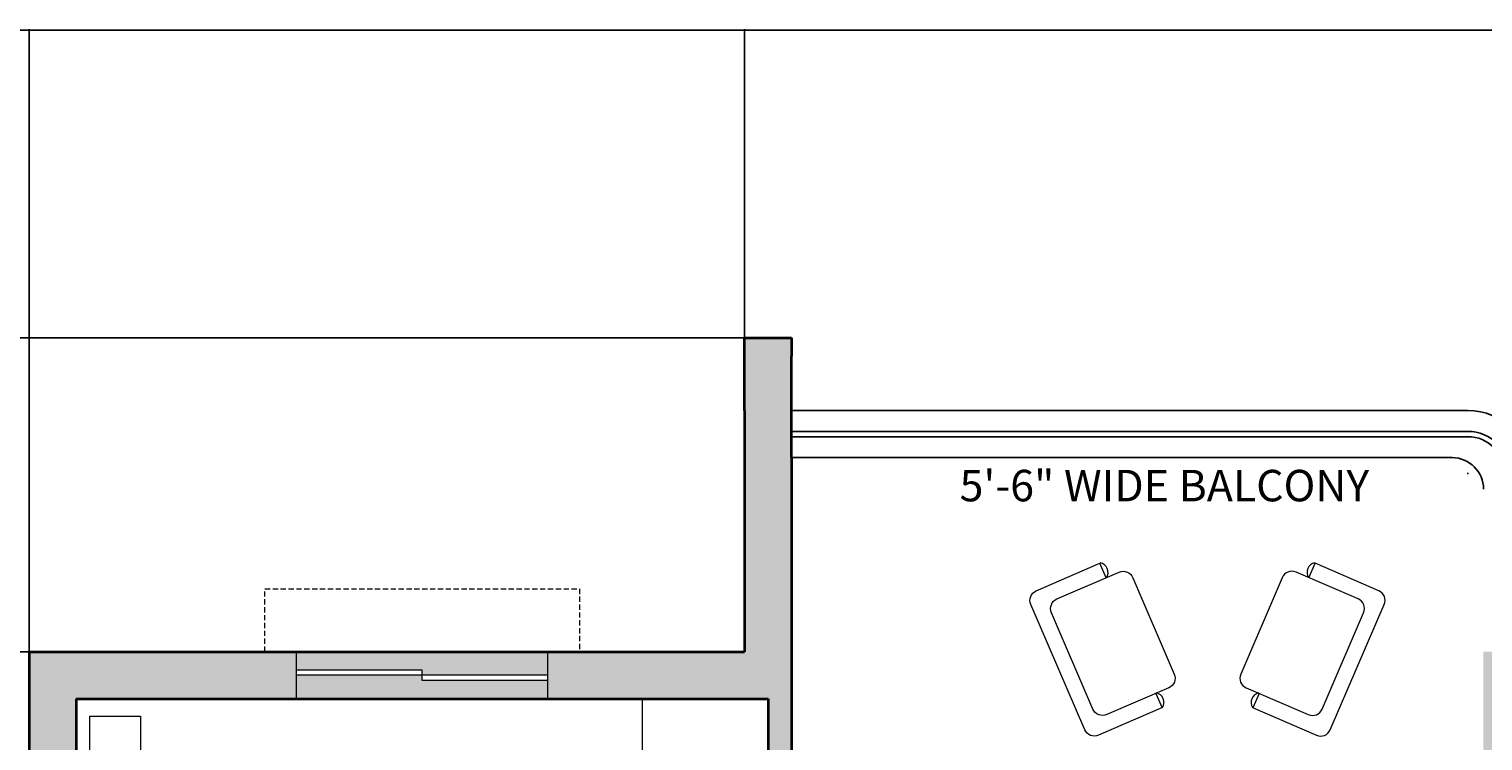
# Model space of a CAD drawing. Units: inches. Extents: x 1693 to 2974, y 2201 to 2965.
# Tile 22 of 24: x 2479 to 2757, y 2829 to 2965. Entities that reach past the tile are written whole.
import ezdxf

# ---------------------------------------------------------------- set-up
doc = ezdxf.new("R2010")
doc.units = ezdxf.units.IN
doc.header["$LTSCALE"] = 2
doc.header["$MEASUREMENT"] = 0
doc.linetypes.add('HIDDEN', pattern=[0.375, 0.25, -0.125])
for name, color, linetype, lineweight in [('A-ANNO-DIMS', 2, 'Continuous', 18), ('A-AREA-IDEN', 7, 'Continuous', 18), ('A-FLOR-CASE', 32, 'Continuous', 18), ('A-FLOR-RAIL', 7, 'Continuous', 25), ('A-FURN', 8, 'Continuous', 18), ('A-GLAZ', 4, 'Continuous', 18), ('A-GLAZ-OVHD', 8, 'HIDDEN', 13), ('A-WALL', 7, 'Continuous', 35)]:
    doc.layers.add(name, color=color, linetype=linetype, lineweight=lineweight)
doc.layers.add('A-GLAZ-PATT', color=141, linetype='Continuous', lineweight=13, true_color=0xadddf7)
doc.layers.add('A-WALL-PATT', color=251, linetype='Continuous', lineweight=13, true_color=0x636466)
doc.styles.get("Standard").update_dxf_attribs({"font": 'arial.ttf'})
doc.dimstyles.get("Standard").update_dxf_attribs({"dimtxt": 0.18, "dimasz": 0.18, "dimexe": 0.18, "dimexo": 0.0625, "dimgap": 0.09, "dimtad": 0, "dimtih": 1, "dimtoh": 1, "dimdec": 1, "dimzin": 0, "dimdsep": 46, "dimlunit": 3, "dimtxsty": 'Standard', "dimcen": 0.09, "dimadec": 0, "dimazin": 0, "dimtfac": 1, "dimtdec": 1, "dimtofl": 0, "dimtmove": 0, "dimatfit": 3, "dimfxl": 1, "dimtolj": 1, "dimtzin": 0, "dimarcsym": 0})

# ---------------------------------------------------------------- blocks, each defined once
blk = doc.blocks.new('NIGHTSTAND')
at = {"ltscale": 2}
blk.add_lwpolyline([(11.51, 0), (0, 0), (0, 9.62), (11.51, 9.62)], close=True, dxfattribs=at)
blk = doc.blocks.new('WINDOW-HOOD-60IN')
at = {"ltscale": 2}
for p, q in [((6, 12), (0, 12)), ((0, 12), (0, 0)), ((60, 12), (6, 12)), ((60, 0), (60, 12)), ((54, 0), (60, 0))]:
    blk.add_line(p, q, dxfattribs=at)
blk = doc.blocks.new('*D81')
at = {"layer": 'A-ANNO-DIMS', "color": 0, "lineweight": -2, "ltscale": 2, "transparency": 16777216}
for p, q in [((1752.34, 2553.91), (1752.34, 2964.96)), ((1752.52, 2964.78), (2332.94, 2964.78)), ((2914.06, 2964.78), (2333.64, 2964.78)), ((2914.24, 2754.97), (2914.24, 2964.96))]:
    blk.add_line(p, q, dxfattribs=at)
at = {"layer": 'A-ANNO-DIMS', "color": 0, "ltscale": 2, "transparency": 16777216}
for points in [[(1752.52, 2964.81), (1752.52, 2964.75), (1752.34, 2964.78)], [(2914.06, 2964.81), (2914.06, 2964.75), (2914.24, 2964.78)]]:
    blk.add_solid(points, dxfattribs=at)
at = {"layer": 'Defpoints', "color": 0, "ltscale": 2, "transparency": 16777216}
for p in [(2914.24, 2964.78), (2914.24, 2754.9), (1752.34, 2553.84)]:
    blk.add_point(p, dxfattribs=at)
at = {"layer": 'A-ANNO-DIMS', "color": 0, "ltscale": 2, "transparency": 16777216, "insert": (2333.29, 2964.78), "char_height": 0.18, "attachment_point": 5}
blk.add_mtext('\\A1;1162', dxfattribs=at)
blk = doc.blocks.new('*D82')
at = {"layer": 'A-ANNO-DIMS', "color": 0, "lineweight": -2, "ltscale": 2, "transparency": 16777216}
for p, q in [((2615.67, 2906.08), (1693.46, 2906.08)), ((1693.64, 2905.9), (1693.64, 2582.94)), ((1693.64, 2259.62), (1693.64, 2582.58)), ((2096.17, 2259.44), (1693.46, 2259.44))]:
    blk.add_line(p, q, dxfattribs=at)
at = {"layer": 'A-ANNO-DIMS', "color": 0, "ltscale": 2, "transparency": 16777216}
for points in [[(1693.61, 2905.9), (1693.67, 2905.9), (1693.64, 2906.08)], [(1693.61, 2259.62), (1693.67, 2259.62), (1693.64, 2259.44)]]:
    blk.add_solid(points, dxfattribs=at)
at = {"layer": 'Defpoints', "color": 0, "ltscale": 2, "transparency": 16777216}
for p in [(1693.64, 2906.08), (2615.74, 2906.08), (2096.24, 2259.44)]:
    blk.add_point(p, dxfattribs=at)
at = {"layer": 'A-ANNO-DIMS', "color": 0, "ltscale": 2, "transparency": 16777216, "insert": (1693.64, 2582.76), "char_height": 0.18, "attachment_point": 5}
blk.add_mtext('\\A1;646.6', dxfattribs=at)
blk = doc.blocks.new('*D91')
at = {"layer": 'A-ANNO-DIMS', "color": 0, "lineweight": -2, "ltscale": 2, "transparency": 16777216}
for p, q in [((2615.67, 2906.08), (1693.46, 2906.08)), ((1693.64, 2905.9), (1693.64, 2876.35)), ((1693.64, 2846.43), (1693.64, 2875.98)), ((2479.17, 2846.25), (1693.46, 2846.25))]:
    blk.add_line(p, q, dxfattribs=at)
at = {"layer": 'A-ANNO-DIMS', "color": 0, "ltscale": 2, "transparency": 16777216}
for points in [[(1693.61, 2905.9), (1693.67, 2905.9), (1693.64, 2906.08)], [(1693.61, 2846.43), (1693.67, 2846.43), (1693.64, 2846.25)]]:
    blk.add_solid(points, dxfattribs=at)
at = {"layer": 'Defpoints', "color": 0, "ltscale": 2, "transparency": 16777216}
for p in [(2615.74, 2906.08), (1693.64, 2846.25), (2479.24, 2846.25)]:
    blk.add_point(p, dxfattribs=at)
at = {"layer": 'A-ANNO-DIMS', "color": 0, "ltscale": 2, "transparency": 16777216, "insert": (1693.64, 2876.17), "char_height": 0.18, "attachment_point": 5}
blk.add_mtext('\\A1;59.82', dxfattribs=at)
blk = doc.blocks.new('*D100')
at = {"layer": 'A-ANNO-DIMS', "color": 0, "lineweight": -2, "ltscale": 2, "transparency": 16777216}
for p, q in [((2615.74, 2906.14), (2615.74, 2964.96)), ((2615.92, 2964.78), (2690.46, 2964.78)), ((2765.56, 2964.78), (2691.02, 2964.78)), ((2765.74, 2880.32), (2765.74, 2964.96))]:
    blk.add_line(p, q, dxfattribs=at)
at = {"layer": 'A-ANNO-DIMS', "color": 0, "ltscale": 2, "transparency": 16777216}
for points in [[(2615.92, 2964.81), (2615.92, 2964.75), (2615.74, 2964.78)], [(2765.56, 2964.81), (2765.56, 2964.75), (2765.74, 2964.78)]]:
    blk.add_solid(points, dxfattribs=at)
at = {"layer": 'Defpoints', "color": 0, "ltscale": 2, "transparency": 16777216}
for p in [(2765.74, 2964.78), (2615.74, 2906.08), (2765.74, 2880.25)]:
    blk.add_point(p, dxfattribs=at)
at = {"layer": 'A-ANNO-DIMS', "color": 0, "ltscale": 2, "transparency": 16777216, "insert": (2690.74, 2964.78), "char_height": 0.18, "attachment_point": 5}
blk.add_mtext('\\A1;150', dxfattribs=at)
blk = doc.blocks.new('*D101')
at = {"layer": 'A-ANNO-DIMS', "color": 0, "lineweight": -2, "ltscale": 2, "transparency": 16777216}
for p, q in [((2479.24, 2846.32), (2479.24, 2964.96)), ((2479.42, 2964.78), (2547.1, 2964.78)), ((2615.56, 2964.78), (2547.87, 2964.78)), ((2615.74, 2846.32), (2615.74, 2964.96))]:
    blk.add_line(p, q, dxfattribs=at)
at = {"layer": 'A-ANNO-DIMS', "color": 0, "ltscale": 2, "transparency": 16777216}
for points in [[(2479.42, 2964.81), (2479.42, 2964.75), (2479.24, 2964.78)], [(2615.56, 2964.81), (2615.56, 2964.75), (2615.74, 2964.78)]]:
    blk.add_solid(points, dxfattribs=at)
at = {"layer": 'Defpoints', "color": 0, "ltscale": 2, "transparency": 16777216}
for p in [(2615.74, 2964.78), (2479.24, 2846.25), (2615.74, 2846.25)]:
    blk.add_point(p, dxfattribs=at)
at = {"layer": 'A-ANNO-DIMS', "color": 0, "ltscale": 2, "transparency": 16777216, "insert": (2547.49, 2964.78), "char_height": 0.18, "attachment_point": 5}
blk.add_mtext('\\A1;136.5', dxfattribs=at)
blk = doc.blocks.new('*D112')
at = {"layer": 'A-ANNO-DIMS', "color": 0, "lineweight": -2, "ltscale": 2, "transparency": 16777216}
for p, q in [((2767.31, 2893.83), (2762.35, 2888.87)), ((2767.49, 2893.83), (2767.31, 2893.83)), ((2753.65, 2880.25), (2753.83, 2880.25)), ((2753.74, 2880.16), (2753.74, 2880.34))]:
    blk.add_line(p, q, dxfattribs=at)
at = {"layer": 'A-ANNO-DIMS', "color": 0, "ltscale": 2, "transparency": 16777216}
blk.add_solid([(2762.33, 2888.89), (2762.37, 2888.85), (2762.22, 2888.74)], dxfattribs=at)
at = {"layer": 'Defpoints', "color": 0, "ltscale": 2, "transparency": 16777216}
for p in [(2762.22, 2888.74), (2753.74, 2880.25)]:
    blk.add_point(p, dxfattribs=at)
at = {"layer": 'A-ANNO-DIMS', "color": 0, "ltscale": 2, "transparency": 16777216, "insert": (2767.99, 2893.83), "char_height": 0.18, "attachment_point": 5}
blk.add_mtext('\\A1;2X R12', dxfattribs=at)

msp = doc.modelspace()

# ---------------------------------------------------------------- hatches: boundary and pattern name
at = {"layer": 'A-GLAZ-PATT', "ltscale": 2}
h = msp.add_hatch(color=256, dxfattribs=at)
h.dxf.hatch_style = 1
h.paths.add_polyline_path([(2656.9702, 2338.2547), (2632.9702, 2338.2547), (2632.9702, 2339.2547), (2608.9702, 2339.2547), (2608.9702, 2334.7547), (2656.9702, 2334.7547)])
h.paths.add_polyline_path([(2656.9702, 2343.7547), (2608.9702, 2343.7547), (2608.9702, 2340.2547), (2632.9702, 2340.2547), (2632.9702, 2339.2547), (2656.9702, 2339.2547)])
h.paths.add_polyline_path([(2775.7544, 2338.2547), (2751.7544, 2338.2547), (2751.7544, 2334.7547), (2775.7544, 2334.7547)])
h.paths.add_polyline_path([(2775.7544, 2343.7547), (2751.7544, 2343.7547), (2751.7544, 2340.2547), (2775.7544, 2340.2547)])
h.paths.add_polyline_path([(2897.7363, 2568.7999), (2893.2363, 2568.7999), (2893.2363, 2520.7999), (2896.7363, 2520.7999), (2896.7363, 2544.7999), (2897.7363, 2544.7999)])
h.paths.add_polyline_path([(2902.2363, 2568.7999), (2898.7363, 2568.7999), (2898.7363, 2544.7999), (2897.7363, 2544.7999), (2897.7363, 2520.7999), (2902.2363, 2520.7999)])
h.paths.add_polyline_path([(2902.2363, 2637.7547), (2898.7363, 2637.7547), (2898.7363, 2613.7547), (2902.2363, 2613.7547)])
h.paths.add_polyline_path([(2896.7363, 2637.7547), (2893.2363, 2637.7547), (2893.2363, 2613.7547), (2896.7363, 2613.7547)])
h.paths.add_polyline_path([(2902.2363, 2748.903), (2899.0477, 2748.903), (2899.0477, 2724.903), (2898.0477, 2724.903), (2898.0477, 2700.903), (2902.2363, 2700.903)])
h.paths.add_polyline_path([(2898.0477, 2748.903), (2893.2363, 2748.903), (2893.2363, 2700.903), (2897.0477, 2700.903), (2897.0477, 2724.903), (2898.0477, 2724.903)])
h.paths.add_polyline_path([(2851.2363, 2846.2547), (2803.2363, 2846.2547), (2803.2363, 2842.7547), (2827.2363, 2842.7547), (2827.2363, 2841.7547), (2851.2363, 2841.7547)])
h.paths.add_polyline_path([(2851.2363, 2840.7547), (2827.2363, 2840.7547), (2827.2363, 2841.7547), (2803.2363, 2841.7547), (2803.2363, 2837.2547), (2851.2363, 2837.2547)])
h.paths.add_polyline_path([(2578.2363, 2846.2547), (2530.2363, 2846.2547), (2530.2363, 2842.7547), (2554.2363, 2842.7547), (2554.2363, 2841.7547), (2578.2363, 2841.7547)])
h.paths.add_polyline_path([(2578.2363, 2840.7547), (2554.2363, 2840.7547), (2554.2363, 2841.7547), (2530.2363, 2841.7547), (2530.2363, 2837.2547), (2578.2363, 2837.2547)])
h.paths.add_polyline_path([(2732.7363, 2812.7547), (2705.1363, 2812.7547), (2705.1363, 2811.7547), (2676.3363, 2811.7547), (2676.3363, 2812.7547), (2648.7363, 2812.7547), (2648.7363, 2808.2547), (2732.7363, 2808.2547)])
h.paths.add_polyline_path([(2732.7363, 2817.2547), (2648.7363, 2817.2547), (2648.7363, 2813.7547), (2676.3363, 2813.7547), (2676.3363, 2812.7547), (2705.1363, 2812.7547), (2705.1363, 2813.7547), (2732.7363, 2813.7547)])
h.paths.add_polyline_path([(2488.2363, 2695.8203), (2484.7878, 2695.8203), (2484.7878, 2671.8203), (2488.2363, 2671.8203)])
h.paths.add_polyline_path([(2482.7878, 2695.8203), (2479.2363, 2695.8203), (2479.2363, 2671.8203), (2482.7878, 2671.8203)])
h.paths.add_polyline_path([(2488.2363, 2572.4371), (2484.7363, 2572.4371), (2484.7363, 2541.4371), (2483.7363, 2541.4371), (2483.7363, 2512.4371), (2488.2363, 2512.4371)])
h.paths.add_polyline_path([(2482.7363, 2541.4371), (2483.7363, 2541.4371), (2483.7363, 2572.4371), (2479.2363, 2572.4371), (2479.2363, 2512.4371), (2482.7363, 2512.4371)])
h.paths.add_polyline_path([(2248.9863, 2706.8449), (2190.9863, 2706.8449), (2190.9863, 2703.3449), (2219.9863, 2703.3449), (2219.9863, 2702.3449), (2248.9863, 2702.3449)])
h.paths.add_polyline_path([(2248.9863, 2701.3449), (2219.9863, 2701.3449), (2219.9863, 2702.3449), (2190.9863, 2702.3449), (2190.9863, 2697.8449), (2248.9863, 2697.8449)])
h.paths.add_polyline_path([(2151.9207, 2293.3449), (2127.9207, 2293.3449), (2127.9207, 2289.8449), (2151.9207, 2289.8449)])
h.paths.add_polyline_path([(2151.9207, 2298.8449), (2127.9207, 2298.8449), (2127.9207, 2295.3449), (2151.9207, 2295.3449)])
h.paths.add_polyline_path([(2084.023, 2293.3449), (2066.023, 2293.3449), (2066.023, 2294.3449), (2048.023, 2294.3449), (2048.023, 2289.8449), (2084.023, 2289.8449)])
h.paths.add_polyline_path([(2084.023, 2298.8449), (2048.023, 2298.8449), (2048.023, 2295.3449), (2066.023, 2295.3449), (2066.023, 2294.3449), (2084.023, 2294.3449)])
h.paths.add_polyline_path([(1966.0781, 2293.3449), (1948.0781, 2293.3449), (1948.0781, 2294.3449), (1930.0781, 2294.3449), (1930.0781, 2289.8449), (1966.0781, 2289.8449)])
h.paths.add_polyline_path([(1966.0781, 2298.8449), (1930.0781, 2298.8449), (1930.0781, 2295.3449), (1948.0781, 2295.3449), (1948.0781, 2294.3449), (1966.0781, 2294.3449)])
h.paths.add_polyline_path([(1787.2363, 2403.1922), (1782.7363, 2403.1922), (1782.7363, 2355.1922), (1786.2363, 2355.1922), (1786.2363, 2379.1922), (1787.2363, 2379.1922)])
h.paths.add_polyline_path([(1791.7363, 2403.1922), (1788.2363, 2403.1922), (1788.2363, 2379.1922), (1787.2363, 2379.1922), (1787.2363, 2355.1922), (1791.7363, 2355.1922)])
h.paths.add_polyline_path([(1786.2363, 2477.5455), (1782.7363, 2477.5455), (1782.7363, 2453.5455), (1786.2363, 2453.5455)])
h.paths.add_polyline_path([(1791.7363, 2477.5455), (1788.2363, 2477.5455), (1788.2363, 2453.5455), (1791.7363, 2453.5455)])
h.paths.add_polyline_path([(1786.2363, 2621.6433), (1782.7363, 2621.6433), (1782.7363, 2585.6433), (1786.2363, 2585.6433)])
h.paths.add_polyline_path([(1791.7363, 2621.6433), (1788.2363, 2621.6433), (1788.2363, 2585.6433), (1791.7363, 2585.6433)])
h.paths.add_polyline_path([(1908.1286, 2706.8449), (1860.1286, 2706.8449), (1860.1286, 2703.3449), (1884.1286, 2703.3449), (1884.1286, 2702.3449), (1908.1286, 2702.3449)])
h.paths.add_polyline_path([(1908.1286, 2701.3449), (1884.1286, 2701.3449), (1884.1286, 2702.3449), (1860.1286, 2702.3449), (1860.1286, 2697.8449), (1908.1286, 2697.8449)])
h.paths.add_polyline_path([(1973.9863, 2706.8449), (1949.9863, 2706.8449), (1949.9863, 2703.3449), (1973.9863, 2703.3449)])
h.paths.add_polyline_path([(1973.9863, 2701.3449), (1949.9863, 2701.3449), (1949.9863, 2697.8449), (1973.9863, 2697.8449)])
h.paths.add_polyline_path([(2112.7363, 2690.3449), (2028.7363, 2690.3449), (2028.7363, 2686.8449), (2056.3363, 2686.8449), (2056.3363, 2685.8449), (2085.1363, 2685.8449), (2085.1363, 2686.8449), (2112.7363, 2686.8449)])
h.paths.add_polyline_path([(2112.7363, 2685.8449), (2085.1363, 2685.8449), (2085.1363, 2684.8449), (2056.3363, 2684.8449), (2056.3363, 2685.8449), (2028.7363, 2685.8449), (2028.7363, 2681.3449), (2112.7363, 2681.3449)])
h.paths.add_polyline_path([(2422.7363, 2640.7547), (2350.7363, 2640.7547), (2350.7363, 2637.2547), (2386.7363, 2637.2547), (2386.7363, 2636.2547), (2422.7363, 2636.2547)])
h.paths.add_polyline_path([(2422.7363, 2635.2547), (2386.7363, 2635.2547), (2386.7363, 2636.2547), (2350.7363, 2636.2547), (2350.7363, 2631.7547), (2422.7363, 2631.7547)])
at = {"layer": 'A-WALL-PATT', "ltscale": 2}
h = msp.add_hatch(color=256, dxfattribs=at)
h.dxf.hatch_style = 1
h.paths.add_polyline_path([(1928.2363, 2733.2161), (1930.9384, 2733.2161), (1930.9384, 2737.2161), (1923.7363, 2737.2161), (1923.7363, 2706.8449), (1908.1286, 2706.8449), (1908.1286, 2697.8449), (1923.7363, 2697.8449), (1923.7363, 2692.8449), (1928.2363, 2692.8449), (1928.2363, 2697.8449), (1949.9863, 2697.8449), (1949.9863, 2706.8449), (1928.2363, 2706.8449)])
h.paths.add_polyline_path([(2004.7363, 2737.2161), (1995.7363, 2737.2161), (1995.7363, 2706.8449), (1985.6374, 2706.8449), (1973.9863, 2706.8449), (1973.9863, 2697.8449), (2000.2363, 2697.8449), (2000.2363, 2686.5348), (2000.3613, 2686.5348), (2000.3613, 2667.0432), (2000.2363, 2601.8449), (1928.2363, 2601.8449), (1928.2363, 2662.8449), (1923.7363, 2662.8449), (1923.7363, 2595.3449), (1928.2363, 2595.3449), (1928.2363, 2597.3449), (2004.7363, 2597.3449), (2004.7363, 2681.3449), (2012.7814, 2681.3449), (2028.7363, 2681.3449), (2028.7363, 2690.3449), (2004.7363, 2690.3449)])
h.paths.add_polyline_path([(2190.9863, 2706.8449), (2184.9863, 2706.8449), (2145.7363, 2706.8449), (2145.7363, 2765.3449), (2145.7363, 2774.5394), (2136.7363, 2774.5394), (2136.7363, 2756.3449), (2136.7363, 2690.3449), (2112.7363, 2690.3449), (2112.7363, 2681.3449), (2136.7363, 2681.3449), (2136.7363, 2597.3449), (2141.2363, 2597.3449), (2141.2363, 2697.8449), (2190.9863, 2697.8449)])
h.paths.add_polyline_path([(1860.1286, 2706.8449), (1782.7363, 2706.8449), (1782.7363, 2621.6433), (1791.7363, 2621.6433), (1791.7363, 2697.8449), (1860.1286, 2697.8449)])
h.paths.add_polyline_path([(1791.7363, 2585.6433), (1782.7363, 2585.6433), (1782.7363, 2562.8449), (1782.7363, 2553.8449), (1752.3363, 2553.8449), (1752.3363, 2544.2586), (1756.3363, 2544.2586), (1756.3363, 2549.3449), (1782.7363, 2549.3449), (1782.7363, 2489.2404), (1782.7363, 2477.5455), (1791.7363, 2477.5455), (1791.7363, 2493.5991), (1791.6113, 2493.5991), (1791.6113, 2513.0907), (1791.6824, 2533.7198, -0.94742783), (1791.7363, 2534.7168), (1791.7363, 2549.3449), (1863.7363, 2549.3449), (1863.7363, 2513.3449), (1866.7363, 2513.3449), (1866.7363, 2549.3449), (1924.7363, 2549.3449), (1924.7363, 2447.3449), (1924.7363, 2442.8449), (1933.7363, 2442.8449), (1933.7363, 2447.3449), (1928.2363, 2447.3449), (1928.2363, 2559.3449), (1923.7363, 2559.3449), (1923.7363, 2553.8449), (1791.7363, 2553.8449), (1791.7363, 2562.8449)])
h.paths.add_polyline_path([(1791.7363, 2442.8449), (1866.7363, 2442.8449), (1866.7363, 2447.3449), (1866.7363, 2483.3449), (1863.7363, 2483.3449), (1863.7363, 2447.3449), (1791.7363, 2447.3449), (1791.7363, 2453.5455), (1782.7363, 2453.5455), (1782.7363, 2447.3449), (1756.3363, 2447.3449), (1756.3363, 2455.7126), (1752.3363, 2455.7126), (1752.3363, 2442.8449), (1782.7363, 2442.8449), (1782.7363, 2403.1922), (1791.7363, 2403.1922)])
h.paths.add_polyline_path([(1930.0781, 2298.8449), (1791.7363, 2298.8449), (1791.7363, 2355.1922), (1782.7363, 2355.1922), (1782.7363, 2289.8449), (1930.0781, 2289.8449)])
h.paths.add_polyline_path([(2624.7363, 2883.2547), (2624.7363, 2902.6165), (2624.7363, 2906.0761), (2615.7363, 2906.0761), (2615.7363, 2892.2547), (2615.7363, 2846.2547), (2578.2363, 2846.2547), (2578.2363, 2837.2547), (2620.2363, 2837.2547), (2620.2363, 2743.2547), (2624.7363, 2743.2547), (2624.7363, 2808.2547), (2648.7363, 2808.2547), (2648.7363, 2817.2547), (2624.7363, 2817.2547)])
h.paths.add_polyline_path([(2530.2363, 2846.2547), (2479.2363, 2846.2547), (2479.2363, 2695.8203), (2488.2363, 2695.8203), (2488.2363, 2700.7547), (2567.2363, 2700.7547), (2567.2363, 2705.2547), (2488.2363, 2705.2547), (2488.2363, 2837.2547), (2530.2363, 2837.2547)])
h.paths.add_polyline_path([(2488.2363, 2487.7547), (2630.2363, 2487.7547, -0.00990191), (2630.2363, 2489.0322), (2630.2363, 2492.2547), (2488.2363, 2492.2547), (2488.2363, 2512.4371), (2479.2363, 2512.4371), (2479.2363, 2334.7547), (2608.9702, 2334.7547), (2608.9702, 2343.7547), (2488.2363, 2343.7547)])
h.paths.add_polyline_path([(2751.7544, 2343.7547), (2672.7363, 2343.7547), (2672.7363, 2409.7547), (2674.7363, 2409.7547), (2674.7363, 2413.7547), (2672.7363, 2413.7547), (2672.7363, 2487.7547), (2732.7363, 2487.7547), (2732.7363, 2413.7547), (2704.7363, 2413.7547), (2704.7363, 2409.7547), (2784.7363, 2409.7547), (2784.7363, 2343.7547), (2775.7544, 2343.7547), (2775.7544, 2334.7547), (2902.2363, 2334.7547), (2902.2363, 2520.7999), (2893.2363, 2520.7999), (2893.2363, 2413.7547), (2856.0145, 2413.7547), (2856.0145, 2409.7547), (2893.2363, 2409.7547), (2893.2363, 2343.7547), (2789.2363, 2343.7547), (2789.2363, 2409.7547), (2819.2363, 2409.7547), (2826.0145, 2409.7547), (2826.0145, 2413.7547), (2789.2363, 2413.7547), (2789.2363, 2492.2547), (2784.7363, 2492.2547), (2784.7363, 2413.7547), (2736.7363, 2413.7547), (2736.7363, 2492.2547), (2672.7363, 2492.2547), (2666.2363, 2492.2547), (2666.2363, 2487.7547), (2668.2363, 2487.7547), (2668.2363, 2343.7547), (2656.9702, 2343.7547), (2656.9702, 2334.7547), (2662.9702, 2334.7547), (2751.7544, 2334.7547)])
h.paths.add_polyline_path([(2902.2363, 2613.7547), (2893.2363, 2613.7547), (2893.2363, 2589.7547), (2785.2363, 2589.7547), (2785.2363, 2661.7547), (2790.2363, 2661.7547), (2790.2363, 2665.2547), (2761.2363, 2665.2547), (2761.2363, 2667.2547), (2756.7363, 2667.2547), (2756.7363, 2661.7547), (2781.2363, 2661.7547), (2781.2363, 2585.7547), (2893.2363, 2585.7547), (2893.2363, 2568.7999), (2902.2363, 2568.7999)])
h.paths.add_polyline_path([(2488.2363, 2671.8203), (2479.2363, 2671.8203), (2479.2363, 2645.2547), (2479.2363, 2623.4598), (2488.2363, 2623.4598), (2488.2363, 2636.2547), (2624.7363, 2636.2547), (2624.7363, 2640.7547), (2603.7363, 2640.7547), (2603.7363, 2700.7547), (2624.7363, 2700.7547), (2624.7363, 2707.2547), (2620.2363, 2707.2547), (2620.2363, 2705.2547), (2597.2363, 2705.2547), (2597.2363, 2700.7547), (2599.2363, 2700.7547), (2599.2363, 2640.7547), (2488.2363, 2640.7547)])
h.paths.add_polyline_path([(2761.2363, 2837.2547), (2803.2363, 2837.2547), (2803.2363, 2846.2547), (2797.2363, 2846.2547), (2765.7363, 2846.2547), (2756.7363, 2846.2547), (2756.7363, 2817.2547), (2732.7363, 2817.2547), (2732.7363, 2808.2547), (2756.7363, 2808.2547), (2756.7363, 2703.2547), (2761.2363, 2703.2547)])
h.paths.add_polyline_path([(2739.7489, 2433.1234), (2786.9181, 2433.1234), (2786.9181, 2455.5122), (2739.7489, 2455.5122)], flags=25)

# ---------------------------------------------------------------- linework, layer by layer
at = {"layer": 'A-FLOR-CASE'}
msp.add_line((2596.2363, 2837.2547), (2596.2363, 2771.2547), dxfattribs=at)
at = {"layer": 'A-FLOR-RAIL', "ltscale": 2}
msp.add_line((2624.7363, 2883.2547), (2750.7363, 2883.2547), dxfattribs=at)
for points in [[(2765.7363, 2846.2547), (2765.7363, 2880.2547, 0.41421356), (2753.7363, 2892.2547), (2624.7363, 2892.2547)], [(2761.7363, 2846.2547), (2761.7363, 2880.2547, 0.41421356), (2753.7363, 2888.2547), (2624.7363, 2888.2547)], [(2760.7363, 2846.2547), (2760.7363, 2880.2547, 0.41421356), (2753.7363, 2887.2547), (2624.7363, 2887.2547)]]:
    msp.add_lwpolyline(points, format="xyb", dxfattribs=at)
msp.add_arc((2750.7363, 2877.2547), 6, 0, 90, dxfattribs=at)
at = {"layer": 'A-FURN', "ltscale": 2}
for p, q in [((2684.735, 2860.3573), (2683.5487, 2863.1128)), ((2723.4297, 2860.3573), (2724.6161, 2863.1128)), ((2694.2279, 2838.3091), (2695.4143, 2835.5536)), ((2713.9368, 2838.3091), (2712.7505, 2835.5536))]:
    msp.add_line(p, q, dxfattribs=at)
for points in [[(2695.5025, 2835.5916), (2683.2803, 2830.3293, -0.41421356), (2680.6524, 2831.3754), (2670.3686, 2855.2607, -0.41421356), (2671.4147, 2857.8885), (2683.5487, 2863.1128)], [(2712.6622, 2835.5916), (2724.8845, 2830.3293, 0.41421356), (2727.5123, 2831.3754), (2737.7961, 2855.2607, 0.41421356), (2736.75, 2857.8885), (2724.6161, 2863.1128)], [(2697.7397, 2841.9985, -0.41421356), (2696.6936, 2839.3707), (2684.8494, 2834.2712, -0.41421356), (2682.2215, 2835.3172), (2674.3105, 2853.6916, -0.41421356), (2675.3565, 2856.3194), (2687.2007, 2861.4189, -0.41421356), (2689.8286, 2860.3729), (2697.7397, 2841.9985)], [(2710.4251, 2841.9985, 0.41421356), (2711.4711, 2839.3707), (2723.3154, 2834.2712, 0.41421356), (2725.9432, 2835.3172), (2733.8543, 2853.6916, 0.41421356), (2732.8082, 2856.3194), (2720.964, 2861.4189, 0.41421356), (2718.3361, 2860.3729), (2710.4251, 2841.9985)]]:
    msp.add_lwpolyline(points, format="xyb", dxfattribs=at)
for centre, start, end in [((2683.2418, 2861.372), 328.302666, 78.285801), ((2724.9229, 2861.372), 101.714199, 211.697334), ((2693.921, 2836.5682), 328.302666, 78.285801), ((2714.2437, 2836.5682), 101.714199, 211.697334)]:
    msp.add_arc(centre, 1.8587, start, end, dxfattribs=at)
at = {"layer": 'A-GLAZ', "ltscale": 2}
for p, q in [((2530.2363, 2837.2547), (2530.2363, 2846.2547)), ((2578.2363, 2837.2547), (2578.2363, 2846.2547)), ((2554.2363, 2842.7547), (2530.2363, 2842.7547)), ((2578.2363, 2841.7547), (2530.2363, 2841.7547)), ((2554.2363, 2840.7547), (2554.2363, 2842.7547)), ((2578.2363, 2840.7547), (2554.2363, 2840.7547))]:
    msp.add_line(p, q, dxfattribs=at)
at = {"layer": 'A-WALL', "ltscale": 2}
for p, q in [((2615.7363, 2892.2547), (2615.7363, 2906.0761)), ((2615.7363, 2906.0761), (2624.7363, 2906.0761)), ((2624.7363, 2906.0761), (2624.7363, 2902.6165)), ((2624.7363, 2883.2547), (2624.7363, 2902.6165)), ((2479.2363, 2846.2547), (2615.7363, 2846.2547)), ((2488.2363, 2837.2547), (2620.2363, 2837.2547))]:
    msp.add_line(p, q, dxfattribs=at)
at = {"layer": 'A-WALL'}
for p, q in [((2615.7363, 2892.2547), (2615.7363, 2846.2547)), ((2624.7363, 2883.2547), (2624.7363, 2817.2547)), ((2479.2363, 2846.2547), (2479.2363, 2645.2547)), ((2488.2363, 2837.2547), (2488.2363, 2705.2547)), ((2620.2363, 2837.2547), (2620.2363, 2743.2547))]:
    msp.add_line(p, q, dxfattribs=at)

# ---------------------------------------------------------------- block references
at = {"layer": 'A-FURN', "rotation": 270.0000000000035}
msp.add_blockref('NIGHTSTAND', (2490.8504, 2833.9797), dxfattribs=at)
at = {"layer": 'A-GLAZ-OVHD', "extrusion": (0, 0, -1), "zscale": -1}
msp.add_blockref('WINDOW-HOOD-60IN', (-2584.2359, 2846.2548), dxfattribs=at)

# ---------------------------------------------------------------- texts
at = {"layer": 'A-AREA-IDEN', "ltscale": 2, "insert": (2656.7788, 2880.9277), "char_height": 6, "attachment_point": 1}
msp.add_mtext_dynamic_manual_height_columns('5\'-6" WIDE BALCONY', width=108.452746, gutter_width=1, heights=[0], dxfattribs=at)

# ---------------------------------------------------------------- dimensions: what is measured, and where the dimension line sits
at = {"layer": 'A-ANNO-DIMS', "ltscale": 2}
for base, p1, p2, override, picture, middle in [((2914.2363, 2964.7761), (1752.3363, 2553.8449), (2914.2363, 2754.903), {"dimdec": 0, "dimlfac": 1, "dimrnd": 0, "dimzin": 0, "dimdsep": 46, "dimlunit": 2}, '*D81', (2333.2863, 2964.7761)), ((2615.7363, 2964.7761), (2479.2363, 2846.2547), (2615.7363, 2846.2547), {"dimdec": 1, "dimlfac": 1, "dimrnd": 0, "dimzin": 0, "dimdsep": 46, "dimlunit": 2}, '*D101', (2547.4863, 2964.7761)), ((2765.7363, 2964.7761), (2615.7363, 2906.0761), (2765.7363, 2880.2547), {"dimdec": 0, "dimlfac": 1, "dimrnd": 0, "dimzin": 0, "dimdsep": 46, "dimlunit": 2}, '*D100', (2690.7363, 2964.7761))]:
    dim = msp.add_linear_dim(base=base, p1=p1, p2=p2, dimstyle='Standard', override=override, dxfattribs=at)
    dim.commit()
    dim.dimension.update_dxf_attribs({"geometry": picture, "text_midpoint": middle})
for base, p1, p2, override, picture, middle in [((1693.6363, 2906.0761), (2096.2363, 2259.4449), (2615.7363, 2906.0761), {"dimdec": 1, "dimlfac": 1, "dimrnd": 0, "dimzin": 0, "dimdsep": 46, "dimlunit": 2}, '*D82', (1693.6363, 2582.7605)), ((1693.6363, 2846.2547), (2615.7363, 2906.0761), (2479.2363, 2846.2547), {"dimdec": 2, "dimlfac": 1, "dimrnd": 0, "dimzin": 0, "dimdsep": 46, "dimlunit": 2}, '*D91', (1693.6363, 2876.1654))]:
    dim = msp.add_linear_dim(base=base, p1=p1, p2=p2, angle=90, dimstyle='Standard', override=override, dxfattribs=at)
    dim.commit()
    dim.dimension.update_dxf_attribs({"geometry": picture, "text_midpoint": middle})
dim = msp.add_radius_dim(center=(2753.7363, 2880.2547), mpoint=(2762.2218, 2888.7398), text='2X <>', dimstyle='Standard', override={"dimdec": 0, "dimlfac": 1, "dimrnd": 0, "dimzin": 0, "dimdsep": 46, "dimlunit": 2}, dxfattribs=at)
dim.commit()
dim.dimension.update_dxf_attribs({"geometry": '*D112', "text_midpoint": (2767.9921, 2893.8308), "dimtype": 164})

doc.saveas('drawing.dxf')
